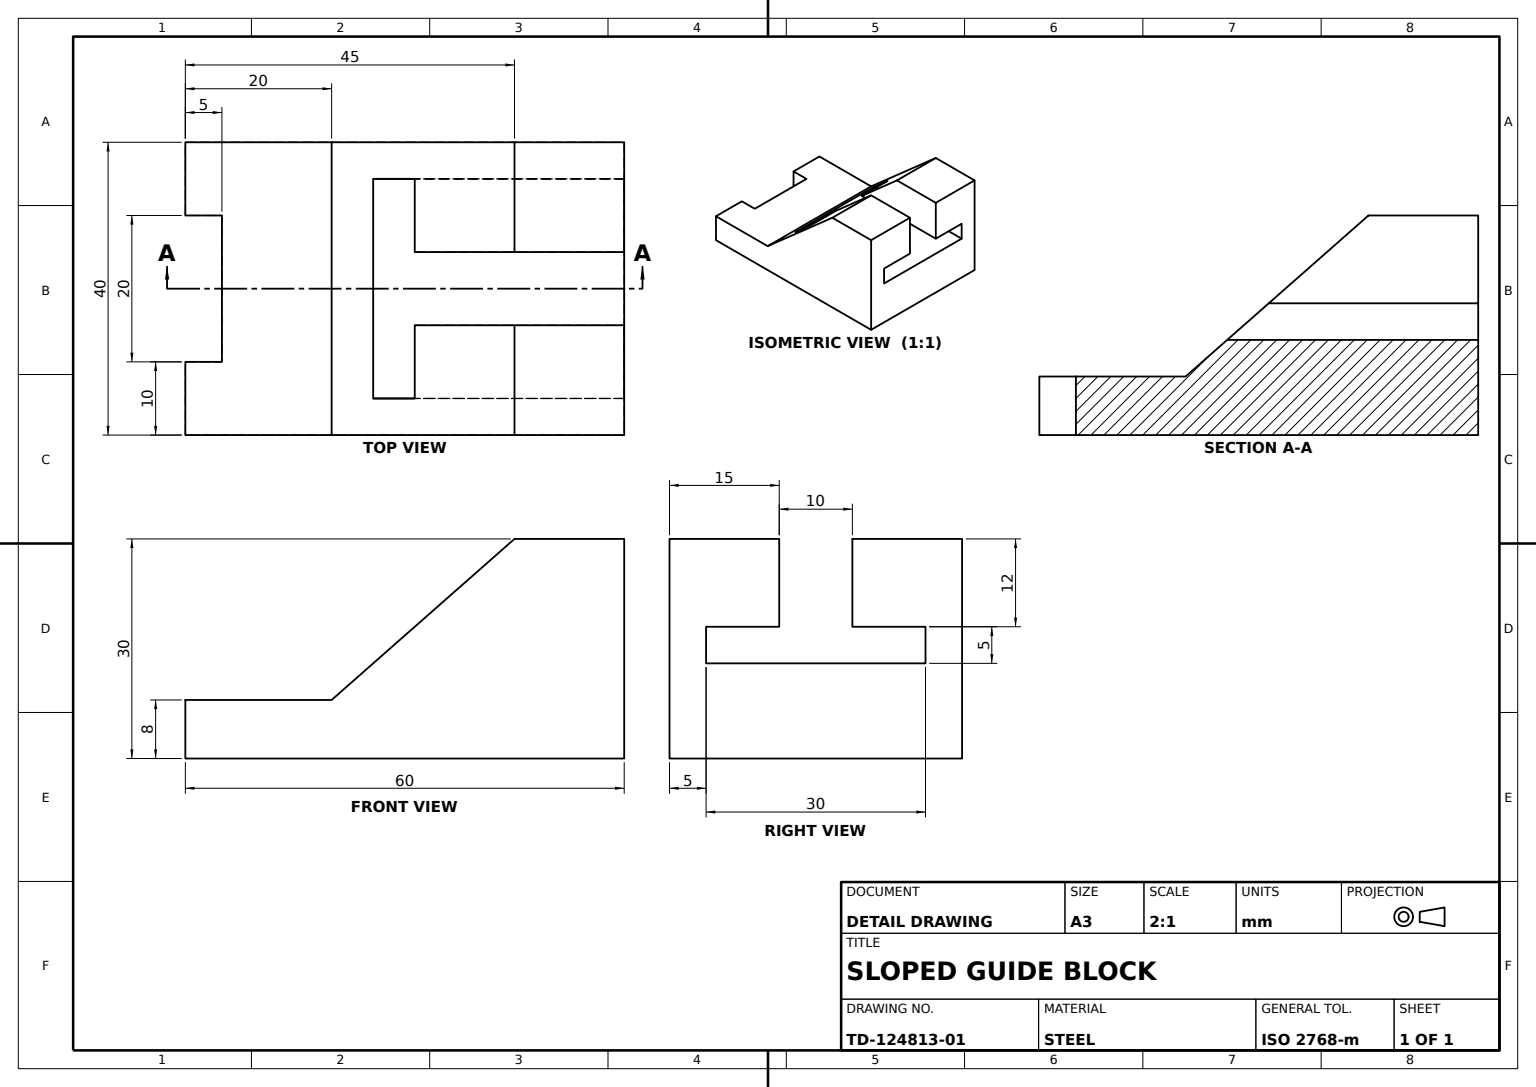
SolidWorks part; units mm, degrees
material "Plain Carbon Steel"
ref_plane "Front Plane" through (0, 0, 0) normal (0, 0, 1) x (1, 0, 0)
ref_plane "Top Plane" through (0, 0, 0) normal (0, 1, 0) x (1, 0, 0)
ref_plane "Right Plane" through (0, 0, 0) normal (1, 0, 0) x (0, 0, -1)
sketch "Base Profile Sketch" plane through (0, 0, 0) normal (0, 0, 1) x (1, 0, 0)
  line L0 (0, 0) -> (60, 0)
  line L1 (60, 0) -> (60, 30)
  line L2 (60, 30) -> (45, 30)
  line L3 (0, 0) -> (0, 8)
  line L4 (0, 8) -> (20, 8)
  line L6 (20, 8) -> (45, 30)
  dimension "D1" = 20
  dimension "D2" = 45
  dimension "D3" = 60
  dimension "D4" = 8
  dimension "D5" = 30
extrude "Angled Base Block" add sketch "Base Profile Sketch" along normal blind 40
sketch "Groove Profile Sketch" plane through (0, 0, 0) normal (-1, 0, 0) x (0, 0, 1)
  line L0 (20, 8) -> (10, 8)
  line L1 (40, 8) -> (0, 8) construction
  line L2 (10, 8) -> (10, 0)
  line L3 (40, 0) -> (0, 0) construction
  line L4 (10, 0) -> (30, 0)
  line L5 (30, 0) -> (30, 8)
  line L6 (30, 8) -> (20, 8)
  line L7 (0, 8) -> (0, 0) construction
  dimension "D1" = 10
extrude "Groove Cut 5mm" cut sketch "Groove Profile Sketch" against normal blind 5
sketch "T-Slot Profile Sketch" plane through (60, 0, 0) normal (1, 0, 0) x (0, 0, -1)
  line L0 (-20, 30) -> (-25, 30)
  line L1 (-40, 30) -> (0, 30) construction
  line L2 (-25, 30) -> (-25, 18)
  line L3 (-20, 30) -> (-15, 30)
  line L4 (-15, 30) -> (-15, 18)
  line L5 (-15, 18) -> (-5, 18)
  line L6 (-5, 18) -> (-5, 13)
  line L7 (-5, 13) -> (-35, 13)
  line L8 (-35, 13) -> (-35, 18)
  line L9 (-35, 18) -> (-25, 18)
  line L10 (0, 0) -> (0, 30) construction
  dimension "D1" = 5
  dimension "D2" = 15
  dimension "D3" = 12
extrude "T-Slot Through Cut" cut sketch "T-Slot Profile Sketch" against normal blind 40
